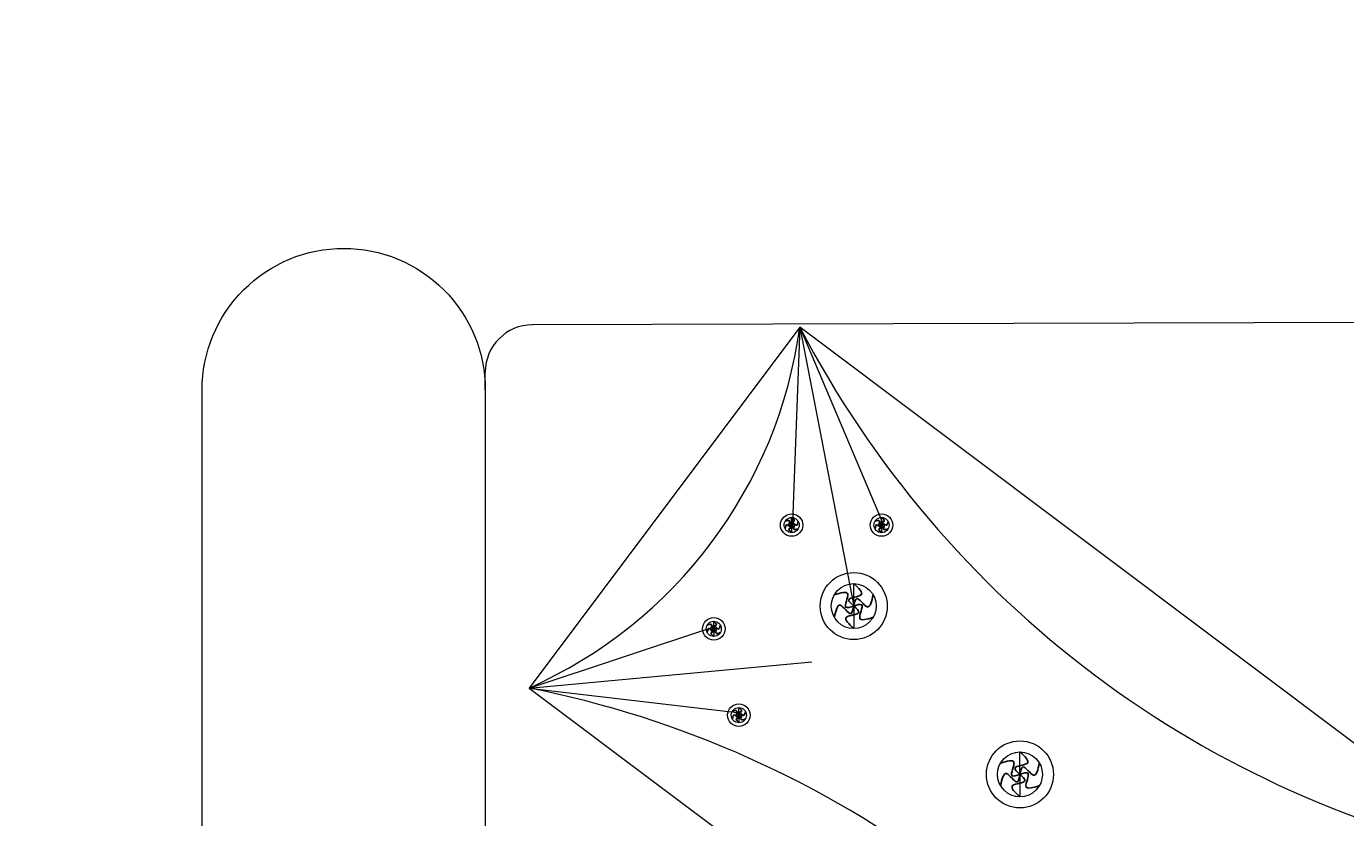
# Model space of a CAD drawing. Units: inches. Extents: x -61 to 1599, y -1316 to 257.
# Tile 100 of 204: x 142 to 170, y -147 to -131. Entities that reach past the tile are written whole.
import ezdxf

# ---------------------------------------------------------------- set-up
doc = ezdxf.new("R2010")
doc.units = ezdxf.units.IN
doc.header["$MEASUREMENT"] = 0
doc.layers.add('A-ANNO-DIMS', color=2, linetype='Continuous', lineweight=18)
doc.layers.add('FURNITURE', color=83, linetype='Continuous', lineweight=18)
doc.layers.add('FUR', color=83, linetype='Continuous')
doc.styles.get("Standard").update_dxf_attribs({"font": 'arial.ttf'})
doc.dimstyles.get("Standard").update_dxf_attribs({"dimtxt": 0.18, "dimasz": 0.18, "dimexe": 0.18, "dimexo": 0.0625, "dimgap": 0.09, "dimtad": 0, "dimtih": 1, "dimtoh": 1, "dimdec": 0, "dimzin": 0, "dimdsep": 46, "dimlunit": 3, "dimtxsty": 'Standard', "dimcen": 0.09, "dimadec": 0, "dimazin": 0, "dimtfac": 1, "dimtdec": 0, "dimtofl": 0, "dimtmove": 0, "dimatfit": 3, "dimfxl": 1, "dimtolj": 1, "dimtzin": 0, "dimarcsym": 0})

# ---------------------------------------------------------------- blocks, each defined once
blk = doc.blocks.new('*U152')
at = {"layer": 'FUR'}
blk.add_open_spline([(0.005, 0.08), (-0.03, 0.048), (-0.098, -0.015), (0.075, -0.018), (0.024, -0.063), (0.005, -0.08)], degree=3, knots=[0, 0, 0, 0, 0.0954578, 0.1898773, 0.2470677, 0.2470677, 0.2470677, 0.2470677], dxfattribs=at)
blk = doc.blocks.new('*U153')
at = {"layer": 'FUR', "transparency": 16777216}
for p, rotation in [((222.173, -79.977), 60), ((222.312, -79.968), 300), ((222.178, -80.056), 120), ((222.25, -80.092), 180), ((222.317, -80.048), 240)]:
    blk.add_blockref('*U152', p, dxfattribs=dict(at, rotation=rotation))
blk.add_blockref('*U152', (222.24, -79.932), dxfattribs=at)
blk = doc.blocks.new('*U154')
at = {"layer": 'FUR'}
blk.add_open_spline([(0.005, 0.08), (-0.03, 0.048), (-0.098, -0.015), (0.075, -0.018), (0.024, -0.063), (0.005, -0.08)], degree=3, knots=[0, 0, 0, 0, 0.0954578, 0.1898773, 0.2470677, 0.2470677, 0.2470677, 0.2470677], dxfattribs=at)
blk = doc.blocks.new('*U155')
at = {"layer": 'FUR', "transparency": 16777216}
for p, rotation in [((222.173, -79.977), 60), ((222.312, -79.968), 300), ((222.178, -80.056), 120), ((222.25, -80.092), 180), ((222.317, -80.048), 240)]:
    blk.add_blockref('*U154', p, dxfattribs=dict(at, rotation=rotation))
blk.add_blockref('*U154', (222.24, -79.932), dxfattribs=at)
blk = doc.blocks.new('*U148')
at = {"layer": 'FUR'}
blk.add_open_spline([(0.005, 0.08), (-0.03, 0.048), (-0.098, -0.015), (0.075, -0.018), (0.024, -0.063), (0.005, -0.08)], degree=3, knots=[0, 0, 0, 0, 0.0954578, 0.1898773, 0.2470677, 0.2470677, 0.2470677, 0.2470677], dxfattribs=at)
blk = doc.blocks.new('*U149')
at = {"layer": 'FUR', "transparency": 16777216}
for p, rotation in [((222.173, -79.977), 60), ((222.312, -79.968), 300), ((222.178, -80.056), 120), ((222.25, -80.092), 180), ((222.317, -80.048), 240)]:
    blk.add_blockref('*U148', p, dxfattribs=dict(at, rotation=rotation))
blk.add_blockref('*U148', (222.24, -79.932), dxfattribs=at)
blk = doc.blocks.new('*U128')
at = {"layer": 'FUR'}
blk.add_open_spline([(0.015, 0.238), (-0.088, 0.143), (-0.292, -0.045), (0.224, -0.053), (0.072, -0.187), (0.015, -0.238)], degree=3, knots=[0, 0, 0, 0, 0.2846533, 0.5662105, 0.736751, 0.736751, 0.736751, 0.736751], dxfattribs=at)
blk = doc.blocks.new('*U129')
at = {"layer": 'FUR', "transparency": 16777216}
blk.add_blockref('*U128', (662.716, -238.357), dxfattribs=at)
for p, rotation in [((662.517, -238.489), 60), ((662.929, -238.463), 300), ((662.531, -238.727), 120), ((662.745, -238.833), 180), ((662.944, -238.702), 240)]:
    blk.add_blockref('*U128', p, dxfattribs=dict(at, rotation=rotation))
blk = doc.blocks.new('*U150')
at = {"layer": 'FUR'}
blk.add_open_spline([(0.005, 0.08), (-0.03, 0.048), (-0.098, -0.015), (0.075, -0.018), (0.024, -0.063), (0.005, -0.08)], degree=3, knots=[0, 0, 0, 0, 0.0954578, 0.1898773, 0.2470677, 0.2470677, 0.2470677, 0.2470677], dxfattribs=at)
blk = doc.blocks.new('*U151')
at = {"layer": 'FUR', "transparency": 16777216}
for p, rotation in [((222.173, -79.977), 60), ((222.312, -79.968), 300), ((222.178, -80.056), 120), ((222.25, -80.092), 180), ((222.317, -80.048), 240)]:
    blk.add_blockref('*U150', p, dxfattribs=dict(at, rotation=rotation))
blk.add_blockref('*U150', (222.24, -79.932), dxfattribs=at)
blk = doc.blocks.new('*U132')
at = {"layer": 'FUR'}
blk.add_open_spline([(0.015, 0.238), (-0.088, 0.143), (-0.292, -0.045), (0.224, -0.053), (0.072, -0.187), (0.015, -0.238)], degree=3, knots=[0, 0, 0, 0, 0.2846533, 0.5662105, 0.736751, 0.736751, 0.736751, 0.736751], dxfattribs=at)
blk = doc.blocks.new('*U133')
at = {"layer": 'FUR', "transparency": 16777216}
blk.add_blockref('*U132', (662.716, -238.357), dxfattribs=at)
for p, rotation in [((662.517, -238.489), 60), ((662.929, -238.463), 300), ((662.531, -238.727), 120), ((662.745, -238.833), 180), ((662.944, -238.702), 240)]:
    blk.add_blockref('*U132', p, dxfattribs=dict(at, rotation=rotation))
blk = doc.blocks.new('SOFA-THREE-SEAT')
for p, q in [((30, 24.442), (6.996, 24.38)), ((12.664, 24.333), (12.509, 20.192)), ((12.664, 24.333), (13.805, 18.423)), ((12.664, 24.333), (14.414, 20.192)), ((6, 23), (5.999, 23.377)), ((12.49, 20.139), (12.49, 20.299)), ((12.49, 20.139), (12.49, 19.979)), ((14.394, 20.139), (14.394, 20.299)), ((14.394, 20.139), (14.394, 19.979)), ((13.805, 18.423), (13.805, 18.899)), ((13.805, 18.423), (13.805, 17.946)), ((6.926, 16.687), (10.859, 17.993)), ((10.84, 17.94), (10.84, 18.1)), ((10.84, 17.94), (10.84, 17.78)), ((6.926, 16.687), (12.92, 17.243)), ((6.926, 16.687), (11.391, 16.164)), ((11.372, 16.112), (11.372, 16.272)), ((11.372, 16.112), (11.372, 15.952)), ((17.327, 14.857), (17.327, 15.334)), ((17.327, 14.857), (17.327, 14.381))]:
    blk.add_line(p, q)
blk.add_lwpolyline([(78, 8.382), (78, 23, -0.414214), (81, 26), (81, 26, -0.414214), (84, 23), (84, 3, -0.414214), (81, 0), (3, 0, -0.414214), (0, 3), (0, 23, -0.414214), (3, 26), (3, 26, -0.414214), (6, 23), (6, 8.382, 0.414214), (9, 5.382), (75, 5.382, 0.414214)], format="xyb", close=True)
blk.add_lwpolyline([(27.729, 13.028), (12.664, 24.333), (6.926, 16.687), (21.991, 5.382)], close=True)
for centre, radius in [((12.49, 20.139), 0.238), ((12.49, 20.139), 0.16), ((14.394, 20.139), 0.238), ((14.394, 20.139), 0.16), ((13.805, 18.423), 0.71), ((13.805, 18.423), 0.476), ((10.84, 17.94), 0.238), ((10.84, 17.94), 0.16), ((11.372, 16.112), 0.238), ((11.372, 16.112), 0.16), ((17.327, 14.857), 0.71), ((17.327, 14.857), 0.476)]:
    blk.add_circle(centre, radius)
for centre, radius, start, end in [((6.999, 23.38), 1, 90.1542, 180.1542), ((2.937, 25.656), 9.816, 293.9742, 352.253), ((31.951, 34.345), 21.731, 207.4316, 258.7956), ((2.703, -4.63), 21.731, 27.4316, 78.7956)]:
    blk.add_arc(centre, radius, start, end)
at = {"xscale": -1, "rotation": 180}
for name, p in [('*U149', (-209.755, -59.873)), ('*U151', (-207.851, -59.873)), ('*U129', (-648.925, -220.172)), ('*U153', (-211.405, -62.072)), ('*U155', (-210.873, -63.9)), ('*U133', (-645.403, -223.738))]:
    blk.add_blockref(name, p, dxfattribs=at)
blk = doc.blocks.new('*D687')
at = {"layer": 'A-ANNO-DIMS', "color": 0, "lineweight": -2, "transparency": 16777216}
for p, q in [((289.418, 181.677), (-61.077, 181.677)), ((-60.897, 181.497), (-60.897, -528.952)), ((-60.897, -1239.765), (-60.897, -529.316)), ((319.64, -1239.945), (-61.077, -1239.945))]:
    blk.add_line(p, q, dxfattribs=at)
at = {"layer": 'A-ANNO-DIMS', "color": 0, "transparency": 16777216}
for points in [[(-60.927, 181.497), (-60.867, 181.497), (-60.897, 181.677)], [(-60.927, -1239.765), (-60.867, -1239.765), (-60.897, -1239.945)]]:
    blk.add_solid(points, dxfattribs=at)
at = {"layer": 'DEFPOINTS', "color": 0, "transparency": 16777216}
for p in [(289.481, 181.677), (-60.897, -1239.945), (319.703, -1239.945)]:
    blk.add_point(p, dxfattribs=at)
at = {"layer": 'A-ANNO-DIMS', "color": 0, "transparency": 16777216, "insert": (-60.897, -529.134), "char_height": 0.18, "attachment_point": 5}
blk.add_mtext('\\A1;1421.6', dxfattribs=at)
blk = doc.blocks.new('*D700')
at = {"layer": 'A-ANNO-DIMS', "color": 0, "lineweight": -2, "transparency": 16777216}
for p, q in [((14.703, -616.882), (14.703, 257.457)), ((179.752, -616.882), (179.752, 257.457)), ((14.883, 257.277), (96.772, 257.277)), ((179.572, 257.277), (97.683, 257.277))]:
    blk.add_line(p, q, dxfattribs=at)
at = {"layer": 'A-ANNO-DIMS', "color": 0, "transparency": 16777216}
for points in [[(14.883, 257.307), (14.883, 257.247), (14.703, 257.277)], [(179.572, 257.307), (179.572, 257.247), (179.752, 257.277)]]:
    blk.add_solid(points, dxfattribs=at)
at = {"layer": 'DEFPOINTS', "color": 0, "transparency": 16777216}
for p in [(179.752, 257.277), (14.703, -616.945), (179.752, -616.945)]:
    blk.add_point(p, dxfattribs=at)
at = {"layer": 'A-ANNO-DIMS', "color": 0, "transparency": 16777216, "insert": (97.227, 257.277), "char_height": 0.18, "attachment_point": 5}
blk.add_mtext('\\A1;165.05', dxfattribs=at)

msp = doc.modelspace()

# ---------------------------------------------------------------- block references
at = {"layer": 'FURNITURE'}
msp.add_blockref('SOFA-THREE-SEAT', (145.375, -161.379), dxfattribs=at)

# ---------------------------------------------------------------- dimensions: what is measured, and where the dimension line sits
at = {"layer": 'A-ANNO-DIMS'}
dim = msp.add_linear_dim(base=(179.7521, 257.2771), p1=(14.7028, -616.9446), p2=(179.7521, -616.9446), dimstyle='Standard', override={"dimdec": 2, "dimlfac": 1, "dimrnd": 0, "dimzin": 0, "dimdsep": 46, "dimlunit": 2}, dxfattribs=at)
dim.commit()
dim.dimension.update_dxf_attribs({"geometry": '*D700', "text_midpoint": (97.2274, 257.2771)})
dim = msp.add_linear_dim(base=(-60.8972, -1239.9446), p1=(289.4807, 181.6771), p2=(319.7028, -1239.9446), angle=90, dimstyle='Standard', override={"dimdec": 1, "dimlfac": 1, "dimrnd": 0, "dimzin": 0, "dimdsep": 46, "dimlunit": 2}, dxfattribs=at)
dim.commit()
dim.dimension.update_dxf_attribs({"geometry": '*D687', "text_midpoint": (-60.8972, -529.1337)})

doc.saveas('drawing.dxf')
